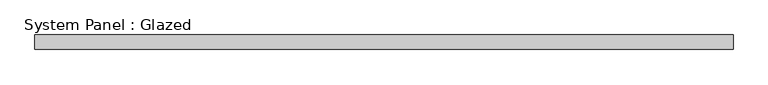
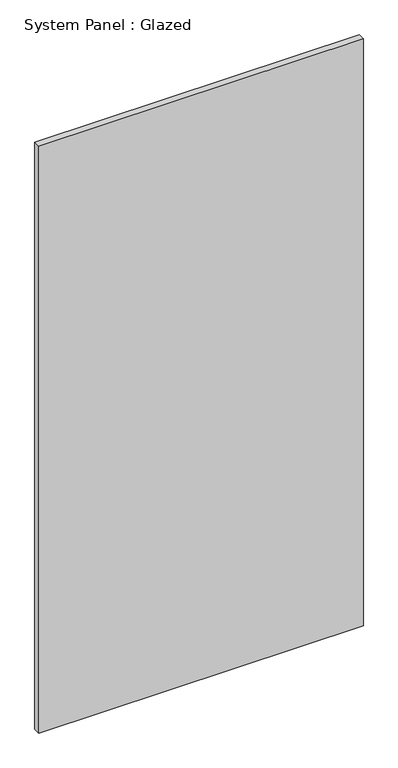
"""IFC4 building model written with IfcOpenShell, lengths in millimetres: plate geometry, System Panel : Glazed."""

from ifc_helpers import new_model, si_unit, origin, origin_with_axes, place, context, project, spatial, polyline, outline, extrude, source, transform, mapped, element, save


def system_panel_glazed_8fc2b39e(model_context):
    return source(origin(), model_context, "Body", "SweptSolid", [
        extrude(outline(polyline([(613.4099999, 19.05), (-613.4099999, 19.05), (-613.4099999, 44.45), (613.4099999, 44.45), (613.4099999, 19.05)])), origin_with_axes(), (0.0, 0.0, 1.0), 2343.15),
    ])


if __name__ == "__main__":
    model = new_model("IFC4")
    model_context = context("Model", 3, world=origin())
    ifc_project = project(units=[si_unit("LENGTHUNIT", "METRE", prefix="MILLI")], contexts=[model_context])
    site = spatial("IfcSite", under=ifc_project)
    building = spatial("IfcBuilding", under=site)
    placement = place(None, origin())
    system_panel_glazed_shape = system_panel_glazed_8fc2b39e(model_context)
    element("IfcPlate", 1, ObjectType="System Panel : Glazed", at=placement, inside=building, context=model_context, shape_type="MappedRepresentation", body=[
        mapped(system_panel_glazed_shape, transform((0.0, 0.0, 0.0), x_axis=(1.0, 0.0, 0.0), y_axis=(0.0, 1.0, 0.0), z_axis=(0.0, 0.0, 1.0))),
    ])
    save(model, "model.ifc")

# Revit data of these elements
# Type "System Panel : Glazed"
#   Construction Type Id = "GSP4R"
#   Analytic Construction = "1/8 in Pilkington single glazing"
#   Visual Light Transmittance = 0.9
#   Solar Heat Gain Coefficient = 0.86
#   Heat Transfer Coefficient (U) = 1.18115 BTU/(h·ft²·°F)
#   Define Thermal Properties by = 1
# Element 1 (IfcPlate, "System Panel : Glazed")
#   Materials on its faces: "Glass"
# Materials
#   "Glass": class "Glass", colour RGB 0 128 192, transparency 0.75, Description = "Soda Lime Glass", Cost = 0
